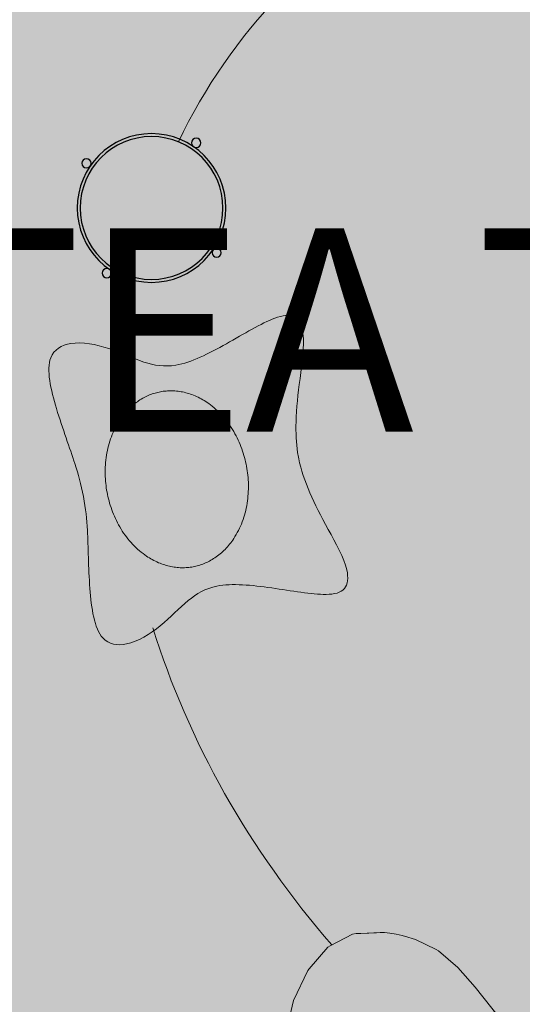
# Model space of a CAD drawing. Units: inches. Extents: x -466983 to 1020, y 324 to 318697.
# Tile 14 of 97: x 752 to 767, y 452 to 482. Entities that reach past the tile are written whole.
import ezdxf

# ---------------------------------------------------------------- set-up
doc = ezdxf.new("R2010")
doc.units = ezdxf.units.IN
doc.header["$MEASUREMENT"] = 0
for name, color, linetype, lineweight in [('A-ANNO-DIMS', 2, 'Continuous', 18), ('A-FLOR-PATT', 252, 'Continuous', 13), ('A-FURN', 8, 'Continuous', 18)]:
    doc.layers.add(name, color=color, linetype=linetype, lineweight=lineweight)
doc.layers.add('CBV_02', color=255, linetype='Continuous')
doc.layers.add('K-Hatch', color=7, linetype='Continuous')
doc.styles.get("Standard").update_dxf_attribs({"font": 'arial.ttf'})
doc.dimstyles.get("Standard").update_dxf_attribs({"dimtxt": 6, "dimasz": 4, "dimexe": 3, "dimexo": 3, "dimgap": 0.09, "dimtad": 0, "dimtih": 1, "dimtoh": 1, "dimdec": 1, "dimzin": 0, "dimdsep": 46, "dimlunit": 3, "dimtxsty": 'Standard', "dimcen": 0.09, "dimadec": 0, "dimazin": 0, "dimtfac": 1, "dimtdec": 1, "dimtofl": 0, "dimtmove": 0, "dimatfit": 3, "dimfxl": 1, "dimtolj": 1, "dimtzin": 0, "dimarcsym": 0})

# ---------------------------------------------------------------- blocks, each defined once
blk = doc.blocks.new('CBV_07')
at = {"layer": 'CBV_02'}
for centre, radius in [((1.45519e-11, 212.4378109452732), 12.43781094527341), ((1.45519e-11, 1.86446e-11), 199.9999999999964), ((-4.36557e-11, -1.77351e-11), 192.0398009950212), ((-212.437810945281, 1.86446e-11), 12.43781094527341), ((212.437810945281, -1.77351e-11), 12.43781094527341), ((-4.36557e-11, -212.4378109452732), 12.43781094527341)]:
    blk.add_circle(centre, radius, dxfattribs=at)
blk = doc.blocks.new('CBV_06')
at = {"layer": 'K-Hatch'}
h = blk.add_hatch(color=256, dxfattribs=at)
h.dxf.hatch_style = 1
h.paths.add_polyline_path([(1007.623919219612, -162.8037901304924), (976.374232667458, -65.00522467460533), (974.5222614408591, -60.86467224506506), (923.3809554458602, 38.00162187329255), (854.3220864886428, 132.5100931947524), (771.0516662640327, 217.2993367493333), (677.2694987420582, 287.0162245334214), (580.7290321753131, 342.4532760775186), (489.1712993668816, 384.41128787848), (414.6868789502657, 413.3806701940782), (369.3663495590927, 429.8539025236807), (337.3779437579125, 440.1607949032459), (302.8898941111865, 450.627018885556), (264.7703254670369, 460.3607313436078), (221.8832241903792, 468.4804353583455), (217.4840165615798, 469.1384541852455), (173.3512318453757, 474.9012920244422), (131.2380269248606, 477.6388986532837), (84.43592055239316, 478.5162570891261), (-21.18851661193878, 478.5845420617116), (-84.4348859316218, 478.5162570891117), (-131.2369923040497, 477.6388986532693), (-173.3522664661657, 474.9012920244279), (-217.4829819407897, 469.1384541852325), (-221.8821895695663, 468.4804353583614), (-264.7692908462292, 460.3607313436078), (-302.8888594903801, 450.6270188855697), (-337.3769091371018, 440.1607949032627), (-369.3653149382831, 429.8539025236967), (-414.687913571062, 413.3806701940782), (-489.1702647460753, 384.4112878784794), (-580.727997554534, 342.4532760775182), (-677.2684641212513, 287.016224533421), (-771.0506316432551, 217.299336749348), (-854.3210518678349, 132.5100931947523), (-923.3799208250532, 38.00162187329153), (-974.5212268200512, -60.86467224508144), (-976.373198046651, -65.00522467462099), (-1007.622884598833, -162.8037901304915), (-1016.399572819664, -252.0315569041262), (-1016.187475556256, -257.5274625777125), (-1002.712574296322, -333.6900379270375), (-999.2528023512159, -339.7756774548897), (-963.8294555040006, -397.2530012106434), (-956.8581805739185, -403.9490670087396), (-946.1912401569826, -410.9368958715785), (-945.1090796062272, -411.6458075578534), (-892.7199681271854, -445.8429323202871), (-879.3112825982488, -451.8892562578833), (-863.7402396036065, -457.7079636201079), (-847.5153162652672, -463.2597388167489), (-832.5629765072194, -467.892770745646), (-820.8407228773971, -470.9469713383587), (-811.5022355638096, -472.6561648949719), (-749.7436509501235, -478.5079801227257), (-742.8861843076988, -478.5845420616969), (-675.1164528635377, -467.1002512151607), (-608.0192249374047, -445.9194942592583), (-540.7130036103011, -420.4678226534015), (-533.4537783415929, -417.8895809303798), (-475.0828679743098, -397.7475499516149), (-450.4835391551242, -390.7507462781742), (-411.1391642374037, -379.9024104451965), (-385.959839948991, -375.7516163159742), (-353.229368988523, -370.5763385811588), (-333.2301869035964, -368.9056247298076), (-297.7038384787113, -366.1945001057087), (-239.8535528132232, -363.6464484829484), (-171.9203512831416, -362.1938408839778), (-95.50739770095436, -361.3475210720644), (-76.22262135388814, -361.3691385733182), (-13.6502694850314, -361.6496303447639), (-21.18851661185556, -361.9269087183784), (13.65130410585698, -361.6496303447637), (76.22365597903189, -361.3691385732987), (95.50843232176425, -361.3475210720499), (171.9193166623488, -362.1938408839924), (239.8545874340225, -363.6464484829484), (297.7048730990744, -366.1945001056892), (333.2153463385341, -368.9044132456776), (353.2283343677303, -370.5763385811734), (386.0094812010862, -375.759629085391), (411.140198858211, -379.9024104451818), (450.3993058632785, -390.7272355487713), (475.0797641119161, -397.7475499516001), (533.4393393600919, -417.8842415422994), (540.7140382311078, -420.4678226534156), (608.0202595582123, -445.9194942592587), (675.1174874843455, -467.1002512151608), (742.8872189285067, -478.5845420617116), (749.7446855709312, -478.5079801227257), (811.5032701846097, -472.6561648949719), (820.8417574981753, -470.9469713383443), (832.5640111280261, -467.8927707456603), (847.5163508860765, -463.259738816748), (863.7412742244078, -457.707963620123), (879.3123172190576, -451.8892562578693), (892.7210027479921, -445.8429323202872), (945.1101142271541, -411.6458075577275), (946.1922747777899, -410.9368958715785), (956.8592151947269, -403.9490670087398), (963.8304901248082, -397.2530012106582), (999.253836972019, -339.7756774548893), (1002.711539675529, -333.6900379270224), (1016.188510177064, -257.527462577709), (1016.399572819664, -252.0315569041411)])
h.paths.add_polyline_path([(474.432091493002, 70.24247514896007), (440.8048463493646, 77.58000584119867), (404.3655018795282, 87.83309793932123), (354.2195010912457, 104.4139308318101), (296.4173064052213, 124.0179256930844), (237.0052417591083, 143.3363652144186), (236.0989139409606, 143.6219205543899), (173.2498390072609, 161.2994514916792), (104.7206958981003, 175.8441506557138), (50.07831894474446, 183.7656277169754), (-6.237828653376141, 188.0444739651632), (-21.18851661185567, 188.7127641286206), (-32.50933737247709, 186.3124438796077), (-104.7196612773207, 175.8441506557137), (-173.2488043864529, 161.2994514916791), (-236.0978793201592, 143.6219205543752), (-237.0042071383106, 143.3363652144165), (-296.4162717844133, 124.0179256930996), (-354.2205357120099, 104.4139308318067), (-404.364467258721, 87.83309793932057), (-440.8038117285569, 77.58000584119856), (-474.4310568721967, 70.24247514895984), (-510.8001823987511, 64.27176482325501), (-524.0473318124533, 62.47661144679296), (-568.5691339483416, 59.7907358578085), (-577.9407609937277, 60.15898080573066), (-570.7894301786835, 66.7702877542913), (-541.1247826875007, 87.83516718090607), (-513.8252783382293, 104.0518135528706), (-490.9022199602167, 116.3348316546901), (-470.501567085256, 126.5030848474575), (-453.3144464057174, 134.5834732719239), (-440.3506478195018, 140.3814882182199), (-432.6158227412204, 143.7026209765454), (-427.2895948783349, 145.7946242280463), (-423.1375757769706, 147.3140928952228), (-410.468729960945, 149.8772378929573), (-379.3307824548831, 154.375769118269), (-338.7494861451014, 159.3137798038201), (-285.0106121184463, 164.8440623421619), (-220.7627298672269, 170.797270408002), (-21.18851661185619, 189.1804127288633), (-6.237828653378585, 188.0444739651632), (32.51037199328522, 186.3124438796075), (50.07831894474282, 183.7656277169755), (220.7616952464316, 170.7972704080169), (285.0095774976543, 164.8440623421628), (338.7504023670155, 159.3137942108383), (379.3318170756569, 154.3757691182548), (410.4697645817553, 149.8772378929571), (423.138594088345, 147.3136775861376), (427.2864910159751, 145.7946242280589), (432.6168573620254, 143.7026209765329), (440.3516824403046, 140.3814882182369), (453.3154810265272, 134.5834732719082), (470.5026017060642, 126.5030848474555), (490.903254581022, 116.3348316546911), (513.8263129590381, 104.0518135528689), (541.1258173083078, 87.83516718090686), (570.7904647994912, 66.7702877542759), (577.941795577851, 60.15898083963367), (568.566030085949, 59.79073585782316), (524.0483664332613, 62.47661144677841), (510.7774931458631, 64.27497970296554)], flags=16)
h = blk.add_hatch(color=256, dxfattribs=at)
h.dxf.hatch_style = 1
h.paths.add_polyline_path([(-412.4365787168098, 142.7921546752039), (-412.5938517189503, 149.4472859239534), (-423.1375757769695, 147.3140928952231), (-427.2895948783371, 145.794624228045), (-432.6158227412198, 143.7026209765462), (-440.350647819501, 140.3814882182197), (-447.8723390510278, 137.0174373274435), (-448.0958186787486, 75.98887565564539), (-440.8038117285577, 77.58000584119874), (-412.2234494581787, 85.62178295929355)])
h.paths.add_polyline_path([(413.3956721956382, 142.5686765830453), (413.2342386251292, 149.3178416264635), (410.4697645817542, 149.8772378929571), (379.3318170756579, 154.3757691182546), (378.2641270243061, 154.5056877103621), (377.9806023147937, 142.5686765830353), (377.8109263829876, 96.61339889887518), (404.3655018795282, 87.83309793932136), (413.6088032993312, 85.23227121955439)])
h.paths.add_polyline_path([(405.3256299791285, 429.6635322970252), (403.2936347338727, 432.8025717950803), (400.7712292308164, 434.6586815048798), (397.6818515310114, 435.9478190179361), (397.4128501237901, 435.9478190179361), (396.6968925322762, 435.9478190179361), (395.6871026344197, 435.9478190179215), (394.6793819781633, 435.9478190179361), (393.6944229794557, 435.9478190179361), (390.6050452796228, 434.6586815048941), (388.0826397765669, 432.8025717950951), (386.0506445313112, 429.6635322970543), (384.7490915686832, 426.5182850741986), (384.7325342462594, 424.2685588886492), (406.7037554884302, 416.282398158631), (406.6271829417563, 426.5182850741984)])
h.paths.add_polyline_path([(-419.2050679706844, 426.739693924741), (-420.5066209333127, 429.8828719059965), (-422.5386161786045, 433.0281191288522), (-425.0589524400528, 434.880090355451), (-428.1503993814221, 436.1712971100787), (-428.4173315470507, 436.1712971100932), (-429.1374276217648, 436.1712971100932), (-430.1451482780212, 436.1712971100787), (-431.1487304511065, 436.1712971100787), (-432.1378279330202, 436.1712971100787), (-435.2272056328184, 434.8800903554364), (-437.7475418942739, 433.0281191288377), (-439.7816063811587, 429.882871906011), (-441.0831593437579, 426.7396939247555), (-441.2611266661435, 403.0452073983812), (-419.0912648160467, 411.6680179526602)])
h = blk.add_hatch(color=256, dxfattribs=at)
h.dxf.hatch_style = 1
h.paths.add_polyline_path([(-296.4162717844122, 124.0179256931005), (-236.3062700041249, 143.5633066007613), (-173.2488043864541, 161.299451491679), (-104.7196612773223, 175.8441506557137), (-32.50933737247766, 186.3124438796076), (-19.56477103674842, 189.0570421156665), (-21.18851661185528, 189.1804127288633), (-220.7627298672269, 170.797270408002), (-285.0106121184475, 164.8440623421629), (-338.1942595667025, 159.3709183261089), (-360.4965454665471, 156.6684888043819), (-379.3307824548866, 154.3757691182691), (-410.4687299609468, 149.877237892957), (-412.5938517189503, 149.4472859239534), (-412.4365787168098, 142.7921546752041), (-412.2234494581786, 85.62178295929355), (-404.3644672587216, 87.83309793932129), (-354.2205357120075, 104.4139308318117)])
h.paths.add_polyline_path([(-447.8723390510278, 137.0174373274435), (-453.3144464057227, 134.5834732719231), (-470.5015670852553, 126.5030848474562), (-490.9022199602147, 116.3348316546909), (-513.8252783382304, 104.0518135528691), (-541.1247826875007, 87.83516718090684), (-570.7894301786836, 66.7702877542907), (-577.9407609937277, 60.15898080573073), (-568.569133948342, 59.79073585780862), (-535.4605149892687, 61.78808608131801), (-514.7554613843324, 63.73577536589507), (-510.8001823987516, 64.27176482325488), (-474.4310568721957, 70.24247514895978), (-448.0958186787486, 75.98887565564539)])
h = blk.add_hatch(color=256, dxfattribs=at)
h.dxf.hatch_style = 1
h.paths.add_polyline_path([(377.9806023147939, 142.568676583047), (377.8109263829876, 96.61339889887523), (354.2195010912438, 104.4139308318117), (296.4173064052192, 124.017925693086), (237.0052417591103, 143.336365214418), (236.0989139409611, 143.6219205543893), (173.2498390072615, 161.299451491679), (104.7206958981005, 175.8441506557137), (50.0783189447435, 183.7656277169755), (-6.237828653376311, 188.0444739651631), (-21.18851661185551, 188.7127641286206), (-32.50933737247744, 186.3124438796076), (-104.7196612773225, 175.8441506557137), (-173.2488043864537, 161.2994514916791), (-236.3062700041244, 143.5633066007612), (-237.0042071382719, 143.3363652144271), (-236.0978793201602, 143.621920554375), (-173.2488043864537, 161.2994514916791), (-104.7196612773222, 175.8441506557137), (-32.50933737247744, 186.3124438796076), (-19.56477103674831, 189.0570421156665), (-6.237828653376197, 188.0444739651631), (32.51037199328499, 186.3124438796076), (50.07831894474373, 183.7656277169755), (220.7616952464342, 170.7972704080166), (285.0095774976544, 164.8440623421629), (338.7504023670157, 159.3137942108386), (378.2641270243062, 154.505687710362)])
h.paths.add_polyline_path([(541.1258173083075, 87.83516718090694), (513.8263129590378, 104.051813552869), (490.9032545810222, 116.3348316546908), (470.5026017060626, 126.5030848474562), (453.3154810265296, 134.5834732719087), (440.3516824403092, 140.3814882182339), (432.6168573620269, 143.7026209765318), (427.2864910159732, 145.7946242280595), (423.1385940883447, 147.3136775861377), (413.2342386251293, 149.3178416264635), (413.3956721956383, 142.5686765830459), (413.6088032993311, 85.23227121955443), (440.8048463493651, 77.58000584119867), (474.4320914930031, 70.24247514895978), (510.7774931458636, 64.27497970296544), (514.7564960049144, 63.73577536591629), (535.4634469349564, 61.78790760318363), (568.566030085949, 59.79073585782315), (577.941795577851, 60.15898083963358), (570.7904647994912, 66.77028775427597)])
for points in [[(472.317326583976, -396.1769955817872), (540.7140382311081, -420.467822653416), (608.0202595582123, -445.9194942592585), (675.1174874843455, -467.1002512151608), (742.8872189285065, -478.5845420617115), (749.7446855709313, -478.5079801227257), (811.5032701846102, -472.6561648949719), (820.8417574981758, -470.9469713383441), (832.5640111280263, -467.8927707456605), (847.5163508860751, -463.2597388167487), (863.7412742244087, -457.7079636201233), (879.3123172190571, -451.8892562578693), (892.7210027479922, -445.8429323202872), (946.2088287105616, -410.9286189052072), (956.8592151947269, -403.9490670087397), (963.8304901248083, -397.2530012106581), (999.2538369720168, -339.7756774548907), (1002.711539675529, -333.6900379270228), (1016.188510177064, -257.5274625777092), (1016.399572819664, -252.0315569041413), (1007.623919219612, -162.8037901304924), (976.3742326674583, -65.00522467460542), (974.5222614408596, -60.86467224506487), (923.3809554458602, 38.00162187329261), (854.3220864886425, 132.5100931947527), (771.051666264033, 217.2993367493327), (677.2694987420582, 287.0162245334213), (580.7290321753135, 342.4532760775182), (489.1712993668806, 384.4112878784799), (414.686878950266, 413.3806701940775), (369.3663495590918, 429.8539025236823), (337.3779437579106, 440.1607949032477), (302.8898941111874, 450.627018885556), (264.7703254670378, 460.3607313436078), (221.8832241903765, 468.4804353583458), (217.4840165615787, 469.1384541852458), (173.3512318453759, 474.9012920244422), (131.2380269248569, 477.6388986532838), (84.43592055239787, 478.5162570891261), (-21.18851661185545, 478.5845420617115), (-84.43488593161965, 478.5162570891116), (-131.2369923040496, 477.6388986532692), (-173.3522664661686, 474.9012920244276), (-217.4829819408005, 469.1384541852312), (-221.8821895695691, 468.4804353583603), (-264.7692908462304, 460.3607313436078), (-302.8888594903801, 450.6270188855705), (-337.3769091371032, 440.1607949032622), (-369.3653149382844, 429.8539025236968), (-414.6879135710587, 413.3806701940775), (-489.1702647460733, 384.4112878784799), (-580.7279975545352, 342.4532760775182), (-677.2684641212508, 287.0162245334213), (-771.0506316432547, 217.2993367493473), (-854.3210518678352, 132.5100931947527), (-923.3799208250529, 38.00162187329261), (-974.5212268200521, -60.86467224507941), (-976.3731980466509, -65.00522467461997), (-1007.622884598833, -162.8037901304924), (-1016.399572819664, -252.0315569041268), (-1016.187475556256, -257.5274625777092), (-1002.712574296322, -333.6900379270373), (-999.2528023512095, -339.7756774548907), (-963.829455504001, -397.2530012106436), (-956.8581805739196, -403.9490670087397), (-946.2077940897543, -410.9286189052072), (-892.7199681271849, -445.8429323202872), (-879.3112825982499, -451.8892562578839), (-863.7402396036014, -457.7079636201087), (-847.5153162652678, -463.2597388167487), (-832.5629765072189, -467.8927707456459), (-820.8407228773976, -470.9469713383587), (-811.5022355638101, -472.6561648949719), (-749.7436509501239, -478.5079801227257), (-742.8861843076993, -478.5845420616969), (-675.1164528635381, -467.1002512151608), (-608.0192249374049, -445.9194942592585), (-540.7130036103008, -420.4678226534015), (-472.320430446347, -396.1769955817872)], [(-441.2611141208436, 403.0468776737834), (-441.0831593437579, 426.7396939247555), (-439.7816063811587, 429.8828719060111), (-437.747541894274, 433.0281191288377), (-435.2272056328184, 434.8800903554365), (-432.1378279330201, 436.1712971100787), (-431.8708957673916, 436.1712971100787), (-431.1487304511065, 436.1712971100787), (-430.1451482780212, 436.1712971100787), (-429.1374276217648, 436.1712971100932), (-428.4173315470507, 436.1712971100932), (-428.1503993814221, 436.1712971100787), (-425.0589524400529, 434.880090355451), (-422.5386161786046, 433.0281191288523), (-420.5066209333126, 429.8828719059965), (-419.2050679706844, 426.739693924741), (-419.0912596830275, 411.6673381542787)], [(384.7325376359404, 424.269019461557), (384.7490915686831, 426.5182850741984), (386.0506445313113, 429.6635322970542), (388.0826397765668, 432.8025717950949), (390.6050452796226, 434.658681504894), (393.6944229794208, 435.9478190179215), (393.9634243866494, 435.9478190179361), (394.6793819781633, 435.9478190179361), (395.6871026344197, 435.9478190179215), (396.6968925322762, 435.9478190179361), (397.4128501237901, 435.9478190179361), (397.6818515310115, 435.9478190179361), (400.7712292308169, 434.6586815048794), (403.2936347338727, 432.8025717950804), (405.3256299791282, 429.663532297025), (406.6271829417564, 426.5182850741984), (406.7037448807277, 416.2838161504187)], [(-510.7565930543751, 64.2789208751201), (-474.4310568721957, 70.24247514895978), (-440.8038117285578, 77.58000584119873), (-404.3644672587215, 87.8330979393213), (-354.2205357120074, 104.4139308318117), (-296.416271784412, 124.0179256931005), (-237.0042071383032, 143.336365214418), (-236.0978793201612, 143.6219205543748), (-173.2488043864541, 161.299451491679), (-104.7196612773223, 175.8441506557137), (-32.5093373724776, 186.3124438796076), (-21.18851661185545, 188.7127641286206), (32.51037199328493, 186.3124438796076), (104.7206958981005, 175.8441506557137), (173.2498390072614, 161.299451491679), (236.0989139409612, 143.6219205543893), (237.0052417591105, 143.336365214418), (296.4173064052193, 124.017925693086), (354.2195010912437, 104.4139308318117), (404.3655018795289, 87.8330979393213), (440.8048463493651, 77.58000584119873), (474.4320914930031, 70.24247514895978), (510.7534891919822, 64.27892087513465)], [(360.4706799466112, 156.6705580459674), (338.1952941875097, 159.3709183261089), (285.0095774976544, 164.8440623421629), (220.7616952464341, 170.7972704080166), (-21.18851661185545, 189.1804127288633), (-220.7627298672269, 170.797270408002), (-285.0106121184472, 164.8440623421629), (-338.1942595667024, 159.3709183261089), (-360.4965454665471, 156.6684888043819)], [(-335.2869751271901, 159.7351048466371), (-379.3307824548865, 154.3757691182691), (-410.4687299609468, 149.877237892957), (-423.1407654824251, 147.3134475580154)], [(423.1397308616323, 147.31344755803), (410.4697645817541, 149.877237892957), (379.3318170756574, 154.3757691182545), (335.2880097479974, 159.7351048466516)], [(-421.539172488683, 147.8990429291152), (-427.2895948783371, 145.794624228045), (-432.6158227412197, 143.7026209765463), (-440.3506478195013, 140.3814882182196), (-453.3144464057222, 134.5834732719231), (-470.5015670852553, 126.5030848474562), (-490.902219960215, 116.3348316546908), (-513.8252783382304, 104.0518135528691), (-541.1247826875006, 87.83516718090686), (-570.7894301786836, 66.77028775429062), (-600.4933932601233, 39.30938256067748)], [(-448.0958191057252, 75.98875905542809), (-447.8723410135826, 137.016901386436)], [(-412.5938410779453, 149.446835641429), (-412.4365787168098, 142.792154675204), (-412.2234468326314, 85.62107867536542)], [(377.810924504116, 96.61289002253035), (377.9806023147939, 142.5686765830469), (378.2640884131724, 154.504062097083)], [(413.2342713512953, 149.3164734209858), (413.3956721956383, 142.5686765830469), (413.6088040798094, 85.23206125570869)], [(600.4944278809307, 39.30938256067748), (570.790464799491, 66.77028775427607), (541.1258173083078, 87.83516718090686), (513.8263129590378, 104.0518135528691), (490.9032545810223, 116.3348316546908), (470.5026017060626, 126.5030848474562), (453.3154810265296, 134.5834732719086), (440.3516824403086, 140.3814882182341), (432.6168573620271, 143.7026209765317), (427.2864910159732, 145.7946242280595), (421.5402071094904, 147.8990429291298)], [(-578.844987703993, 59.32515649918059), (-574.9548135073309, 58.88854652283772)], [(-577.942798369022, 60.159060861537), (-568.5691339483419, 59.79073585780861), (-524.0473318124531, 62.47661144679296), (-499.7378815664742, 65.77084406440554)], [(-514.766783263487, 63.73471033592068), (-535.4881685855325, 61.78548475440766)], [(-440.646549367444, 77.62345991465554), (-440.8038117285578, 77.58000584119873)], [(440.8048463493651, 77.58000584119873), (440.757253792708, 77.59242129075572)], [(499.7389161872742, 65.77084406440554), (524.0483664332605, 62.47661144677841), (568.566030085949, 59.79073585782316), (577.9438329898294, 60.15906086155155)], [(535.4892032063398, 61.78548475440766), (514.7678178842943, 63.73471033592068)], [(574.9558481281455, 58.88854652283772), (578.8460223248002, 59.32515649918059)], [(-592.1026185965856, 47.06696929648751), (-603.9552344468647, 32.76230215735268)], [(603.9562690676429, 32.76230215736723), (592.1036532173929, 47.06696929647296)], [(-450.4485467980666, -390.7410979144188), (-411.1391642374037, -379.9024104451965), (-350.0344599674099, -369.8293423657451)], [(-385.906832240511, -375.7432348412986), (-353.2293689885228, -370.5763385811588), (-293.7324654370423, -365.6060202724475)], [(-333.1597947685914, -368.9002528900601), (-297.1508525502977, -366.152300053247), (-234.6494102043616, -362.7152897656779)], [(-297.7323094381827, -366.1957541267329), (-239.8535528132234, -363.6464484829485), (-171.9203512831409, -362.1938408839778), (-95.50739770095606, -361.3475210720644), (-14.2855266543811, -361.4385677021928)], [(-76.42899020453842, -361.3682134879927), (-13.65026948503146, -361.6496303447639), (-21.18851661185545, -361.9269087183784), (13.65130410583879, -361.6496303447639), (76.43002482534575, -361.3682134879927)], [(14.28656127518116, -361.4385677021783), (95.5084323217634, -361.3475210720499), (171.9193166623481, -362.1938408839924), (239.8545874340234, -363.6464484829485), (297.73334405899, -366.1957541267329)], [(234.6504448251689, -362.7152897656633), (297.1518871711051, -366.1523000532616), (333.1608293893987, -368.9002528900601)], [(293.7335000578496, -365.6060202724475), (353.22833436773, -370.5763385811733), (385.9057976197109, -375.7432348412986)], [(350.0354945882173, -369.8293423657451), (411.1401988582111, -379.9024104451819), (450.4495814188739, -390.7410979144188)], [(-533.4416886490762, -417.8854091441317), (-475.0828679743099, -397.7475499516149), (-408.2980955288694, -378.7519121189398)], [(408.2991301496694, -378.7519121189398), (475.079764111917, -397.7475499516004), (533.4427232698836, -417.8854091441462)], [(-892.7199681271849, -445.8429323202872), (-902.4619575515788, -439.5834764985193), (-946.1912401569826, -410.9368958715785), (-956.8581805739196, -403.9490670087397)], [(892.7210027479922, -445.8429323202872), (902.4629921723862, -439.5834764985338), (946.1922747777899, -410.9368958715785), (956.8592151947269, -403.9490670087397)]]:
    blk.add_lwpolyline(points)
blk = doc.blocks.new('CBV_12')
at = {"ltscale": 200}
blk.add_open_spline([(-9.313226e-10, -313.6689856333542), (34.47199597302824, -314.3318554564612), (96.50876406778117, -318.8139389617718), (240.3265217448352, -345.3180849059718), (392.3031104528345, -352.0678919447819), (421.2341347071342, -269.3013594668591), (382.8255782761844, -170.6823182621738), (322.4239674016135, -90.58104975993047), (290.3339154102141, -2.882590101566165), (331.4904042299604, 138.7749991867458), (383.1127528108191, 271.9643652962404), (379.7935919561423, 336.8141777501441), (318.1455534129636, 354.8965399071458), (203.6221743698698, 315.0004339051084), (98.05609517812265, 283.4114430824411), (29.99349829379935, 273.6171620629611), (-29.99349829589482, 273.6171620629611), (-98.0560951801017, 283.4114430824411), (-203.6221743717324, 315.0004339051084), (-318.145553412498, 354.8965399071458), (-379.7935919559095, 336.8141777501441), (-383.1127528080251, 271.9643652962404), (-331.4904042297276, 138.7749991867458), (-290.3339154145215, -2.882590101566165), (-322.4239674060373, -90.58104975993047), (-382.8255782806082, -170.6823182621738), (-421.2341347067849, -269.3013594668591), (-392.3031104524853, -352.0678919447819), (-240.326521744486, -345.3180849059718), (-96.50876406743193, -318.8139389617718), (-34.471995972679, -314.3318554564612), (-9.313226e-10, -313.6689856333542)], degree=3, knots=[-0.0401029303072623, -0.0401029303072623, -0.0401029303072623, -0.0401029303072623, 0.4782524944232491, 1.206298609480416, 1.890774805552385, 2.364182384251211, 2.955896546893398, 3.541722974063392, 4.084202277006428, 4.791751260435608, 5.498504468228412, 5.918342864309894, 6.332195342449451, 6.974587155334092, 7.603872125826861, 8.123730840629252, 8.249353082176581, 8.8948340385263, 9.524119009019069, 10.16651082190371, 10.58036330004326, 11.00020169612475, 11.70695490391755, 12.41450388734673, 12.95698319028977, 13.54280961745976, 14.13452378010195, 14.60793135880077, 15.29240755487274, 16.02045366992991, 16.53880909466042, 16.53880909466042, 16.53880909466042, 16.53880909466042], dxfattribs=at)
blk.add_rational_spline([(-9.313226e-10, 132.1501473757671), (-239.4450891335728, 132.1501473757671), (-239.4450891335728, -58.68292919226224), (-239.4450891335728, -249.5160057604662), (-9.313226e-10, -249.5160057604662), (239.4450891314773, -249.5160057604662), (239.4450891314773, -58.68292919226224), (239.4450891314773, 132.1501473757671), (-9.313226e-10, 132.1501473757671)], [1, 0.7071067811865476, 1, 0.7071067811865476, 1, 0.7071067811865476, 1, 0.7071067811865476, 1], degree=2, knots=[0, 0, 0, 1.018498484469714, 1.018498484469714, 2.036996968939431, 2.036996968939431, 3.055495453409146, 3.055495453409146, 4.073993937878862, 4.073993937878862, 4.073993937878862])
blk = doc.blocks.new('Garden Sofa')
at = {"extrusion": (0, 0, -1)}
for start_param, end_param in [(9.234639352962448, 10.28481875168741), (8.92175969868659, 9.026940301606375), (8.07079352439746, 8.538067434615327)]:
    blk.add_ellipse((2450.434344520113, 828.9172181338074), major_axis=(18.680571335226, -14.92282860552713), ratio=0.8335261636002053, start_param=start_param, end_param=end_param, dxfattribs=at)
at = {"xscale": -0.0109740885734132, "yscale": 0.0109740885734132, "zscale": 0.0109740885734132}
for name, p, rotation in [('CBV_07', (2428.94679886318, 838.6756627513653), 235.5267845499325), ('CBV_12', (2430.325331439862, 830.785541132772), 280.5267845499334), ('CBV_06', (2441.681283390746, 808.0370618939298), 148.8828363109627)]:
    blk.add_blockref(name, p, dxfattribs=dict(at, rotation=rotation))
blk = doc.blocks.new('*D113')
at = {"layer": 'A-ANNO-DIMS', "color": 0, "lineweight": -2, "transparency": 16777216}
for p, q in [((704.7099345407843, 504.6522237351473), (709.5248847709719, 509.4132675549068)), ((710.2041170385384, 504.4596180389745), (736.3194883324882, 478.0485582412536)), ((736.4502266725144, 472.5525555338968), (741.2651769027019, 477.3135993536564)), ((739.1319487513783, 475.2042540394889), (741.9444091702684, 472.359949837724)), ((741.9444091702684, 472.359949837724), (745.9444091702684, 472.359949837724))]:
    blk.add_line(p, q, dxfattribs=at)
at = {"layer": 'A-ANNO-DIMS', "color": 0, "transparency": 16777216}
for points in [[(710.6781677388324, 504.9283614421228), (709.7300663382443, 503.9908746358262), (707.3916566196483, 507.3039222407393)], [(736.7935390327824, 478.5173016444019), (735.8454376321941, 477.5798148381053), (739.1319487513783, 475.2042540394889)]]:
    blk.add_solid(points, dxfattribs=at)
at = {"layer": 'Defpoints', "color": 0, "transparency": 16777216}
for p in [(702.5767063894607, 502.5428784209798), (739.1319487513783, 475.2042540394889), (734.3169985211908, 470.4432102197293)]:
    blk.add_point(p, dxfattribs=at)
at = {"layer": 'A-ANNO-DIMS', "color": 0, "transparency": 16777216, "insert": (783.5016670147431, 472.359949837724), "char_height": 6, "attachment_point": 5}
blk.add_mtext('\\A1;TEA TABLE SET 45', dxfattribs=at)

msp = doc.modelspace()

# ---------------------------------------------------------------- hatches: boundary and pattern name
at = {"layer": 'A-FLOR-PATT', "transparency": 33554661}
h = msp.add_hatch(color=256, dxfattribs=at)
h.dxf.hatch_style = 1
h.set_gradient(color1=(19, 155, 72), color2=(0, 107, 0), name='CYLINDER')
h.paths.add_polyline_path([(813.8056775209042, 503.9377328184218), (730.8056775209043, 503.9377328184218), (730.8056775209043, 424.9377328184218), (612.8056775209042, 424.9377328184218), (612.8056775209042, 415.9377328184218), (442.8056775209042, 415.9377328184218), (442.8056775209042, 368.9377328184219), (813.8056775209042, 368.9377328184219)])
h.paths.add_polyline_path([(771.7959187717115, 407.069553802904), (783.7959187717115, 407.069553802904), (783.7959187717115, 371.069553802904), (771.7959187717115, 371.069553802904)], flags=16)
h.paths.add_polyline_path([(755.7959187717115, 407.069553802904), (755.7959187717115, 371.069553802904), (743.7959187717114, 371.069553802904), (743.7959187717114, 407.069553802904)], flags=16)
h.paths.add_polyline_path([(769.7959187717115, 404.069553802904), (769.7959187717115, 374.069553802904), (757.7959187717115, 374.069553802904), (757.7959187717115, 404.069553802904)], flags=16)
h.paths.add_polyline_path([(785.7959187717114, 404.069553802904), (797.7959187717114, 404.069553802904), (797.7959187717114, 374.069553802904), (785.7959187717114, 374.069553802904)], flags=16)
h.paths.add_polyline_path([(741.7959187717115, 404.069553802904), (741.7959187717115, 374.069553802904), (729.7959187717115, 374.069553802904), (729.7959187717115, 404.069553802904)], flags=16)
h.paths.add_polyline_path([(799.7959187717115, 407.069553802904), (811.7959187717115, 407.069553802904), (811.7959187717115, 371.069553802904), (799.7959187717115, 371.069553802904)], flags=16)
h.paths.add_polyline_path([(727.7959187717115, 407.069553802904), (727.7959187717115, 371.069553802904), (715.7959187717115, 371.069553802904), (715.7959187717115, 407.069553802904)], flags=16)
h.paths.add_polyline_path([(713.7959187717115, 404.069553802904), (713.7959187717115, 374.069553802904), (701.7959187717115, 374.069553802904), (701.7959187717115, 404.069553802904)], flags=16)
h.paths.add_polyline_path([(699.7959187717115, 407.069553802904), (699.7959187717115, 371.069553802904), (687.7959187717115, 371.069553802904), (687.7959187717115, 407.069553802904)], flags=16)
h.paths.add_polyline_path([(685.7959187717114, 404.069553802904), (685.7959187717114, 374.069553802904), (673.7959187717115, 374.069553802904), (673.7959187717115, 404.069553802904)], flags=16)
h.paths.add_polyline_path([(671.7959187717115, 407.069553802904), (671.7959187717115, 371.069553802904), (659.7959187717115, 371.069553802904), (659.7959187717115, 407.069553802904)], flags=16)
h.paths.add_polyline_path([(657.7959187717115, 404.069553802904), (657.7959187717115, 374.069553802904), (645.7959187717115, 374.069553802904), (645.7959187717115, 404.069553802904)], flags=16)
h.paths.add_polyline_path([(643.7959187717114, 407.069553802904), (643.7959187717114, 371.069553802904), (631.7959187717114, 371.069553802904), (631.7959187717114, 407.069553802904)], flags=16)
h.paths.add_polyline_path([(629.7959187717115, 404.069553802904), (629.7959187717115, 374.069553802904), (617.7959187717115, 374.069553802904), (617.7959187717115, 404.069553802904)], flags=16)
h.paths.add_polyline_path([(615.7959187717115, 407.069553802904), (615.7959187717115, 371.069553802904), (603.7959187717115, 371.069553802904), (603.7959187717115, 407.069553802904)], flags=16)
h.paths.add_polyline_path([(601.7959187717115, 404.069553802904), (601.7959187717115, 374.069553802904), (589.7959187717114, 374.069553802904), (589.7959187717114, 404.069553802904)], flags=16)
at = {"layer": 'A-FLOR-PATT'}
h = msp.add_hatch(dxfattribs=at)
h.set_pattern_fill('GRASS', color=256, scale=6)
h.set_pattern_definition([(90, (-1212.413693079869, -290.0350025265127), (-4.242640685999999, 4.242640685999999), [1.125, -7.360281377999999]), (45, (-1212.413693079869, -290.0350025265127), (-4.242640687119285, 4.242640687119285), [1.125, -4.875]), (135, (-1212.413693079869, -290.0350025265127), (-4.242640687119285, -4.242640687119284), [1.125, -4.875])])
h.paths.add_polyline_path([(813.8056775209042, 503.9377328184218), (730.8056775209043, 503.9377328184218), (730.8056775209043, 424.9377328184218), (612.8056775209042, 424.9377328184218), (612.8056775209042, 415.9377328184218), (442.8056775209042, 415.9377328184218), (442.8056775209042, 368.9377328184219), (813.8056775209042, 368.9377328184219)])
h.paths.add_polyline_path([(589.7959187717114, 404.069553802904), (601.7959187717115, 404.069553802904), (601.7959187717115, 374.069553802904), (589.7959187717114, 374.069553802904)], flags=16)
h.paths.add_polyline_path([(603.7959187717115, 407.069553802904), (615.7959187717115, 407.069553802904), (615.7959187717115, 371.069553802904), (603.7959187717115, 371.069553802904)], flags=16)
h.paths.add_polyline_path([(617.7959187717115, 404.069553802904), (629.7959187717115, 404.069553802904), (629.7959187717115, 374.069553802904), (617.7959187717115, 374.069553802904)], flags=16)
h.paths.add_polyline_path([(631.7959187717114, 407.069553802904), (643.7959187717114, 407.069553802904), (643.7959187717114, 371.069553802904), (631.7959187717114, 371.069553802904)], flags=16)
h.paths.add_polyline_path([(645.7959187717115, 404.069553802904), (657.7959187717115, 404.069553802904), (657.7959187717115, 374.069553802904), (645.7959187717115, 374.069553802904)], flags=16)
h.paths.add_polyline_path([(659.7959187717115, 407.069553802904), (671.7959187717115, 407.069553802904), (671.7959187717115, 371.069553802904), (659.7959187717115, 371.069553802904)], flags=16)
h.paths.add_polyline_path([(673.7959187717115, 404.069553802904), (685.7959187717114, 404.069553802904), (685.7959187717114, 374.069553802904), (673.7959187717115, 374.069553802904)], flags=16)
h.paths.add_polyline_path([(687.7959187717115, 407.069553802904), (699.7959187717115, 407.069553802904), (699.7959187717115, 371.069553802904), (687.7959187717115, 371.069553802904)], flags=16)
h.paths.add_polyline_path([(701.7959187717115, 404.069553802904), (713.7959187717115, 404.069553802904), (713.7959187717115, 374.069553802904), (701.7959187717115, 374.069553802904)], flags=16)
h.paths.add_polyline_path([(715.7959187717115, 407.069553802904), (727.7959187717115, 407.069553802904), (727.7959187717115, 371.069553802904), (715.7959187717115, 371.069553802904)], flags=16)
h.paths.add_polyline_path([(729.7959187717115, 404.069553802904), (741.7959187717115, 404.069553802904), (741.7959187717115, 374.069553802904), (729.7959187717115, 374.069553802904)], flags=16)
h.paths.add_polyline_path([(743.7959187717114, 407.069553802904), (755.7959187717115, 407.069553802904), (755.7959187717115, 371.069553802904), (743.7959187717114, 371.069553802904)], flags=16)
h.paths.add_polyline_path([(757.7959187717115, 404.069553802904), (769.7959187717115, 404.069553802904), (769.7959187717115, 374.069553802904), (757.7959187717115, 374.069553802904)], flags=16)
h.paths.add_polyline_path([(771.7959187717115, 407.069553802904), (783.7959187717115, 407.069553802904), (783.7959187717115, 371.069553802904), (771.7959187717115, 371.069553802904)], flags=16)
h.paths.add_polyline_path([(785.7959187717114, 404.069553802904), (797.7959187717114, 404.069553802904), (797.7959187717114, 374.069553802904), (785.7959187717114, 374.069553802904)], flags=16)
h.paths.add_polyline_path([(799.7959187717115, 407.069553802904), (811.7959187717115, 407.069553802904), (811.7959187717115, 371.069553802904), (799.7959187717115, 371.069553802904)], flags=16)

# ---------------------------------------------------------------- block references
at = {"layer": 'A-FURN'}
msp.add_blockref('Garden Sofa', (-1672.699650965823, -362.7106367544016), dxfattribs=at)

# ---------------------------------------------------------------- dimensions: what is measured, and where the dimension line sits
at = {"layer": 'A-ANNO-DIMS'}
dim = msp.add_linear_dim(base=(739.1319487513783, 475.2042540394889), p1=(702.5767063894607, 502.5428784209797), p2=(734.3169985211907, 470.4432102197293), angle=314.6774666770457, text='TEA TABLE SET <>', dimstyle='Standard', override={"dimdec": 0, "dimlfac": 1, "dimrnd": 0, "dimzin": 0, "dimdsep": 46, "dimlunit": 2}, dxfattribs=at)
dim.commit()
dim.dimension.update_dxf_attribs({"geometry": '*D113', "text_midpoint": (783.5016670147431, 472.359949837724)})

doc.saveas('drawing.dxf')
